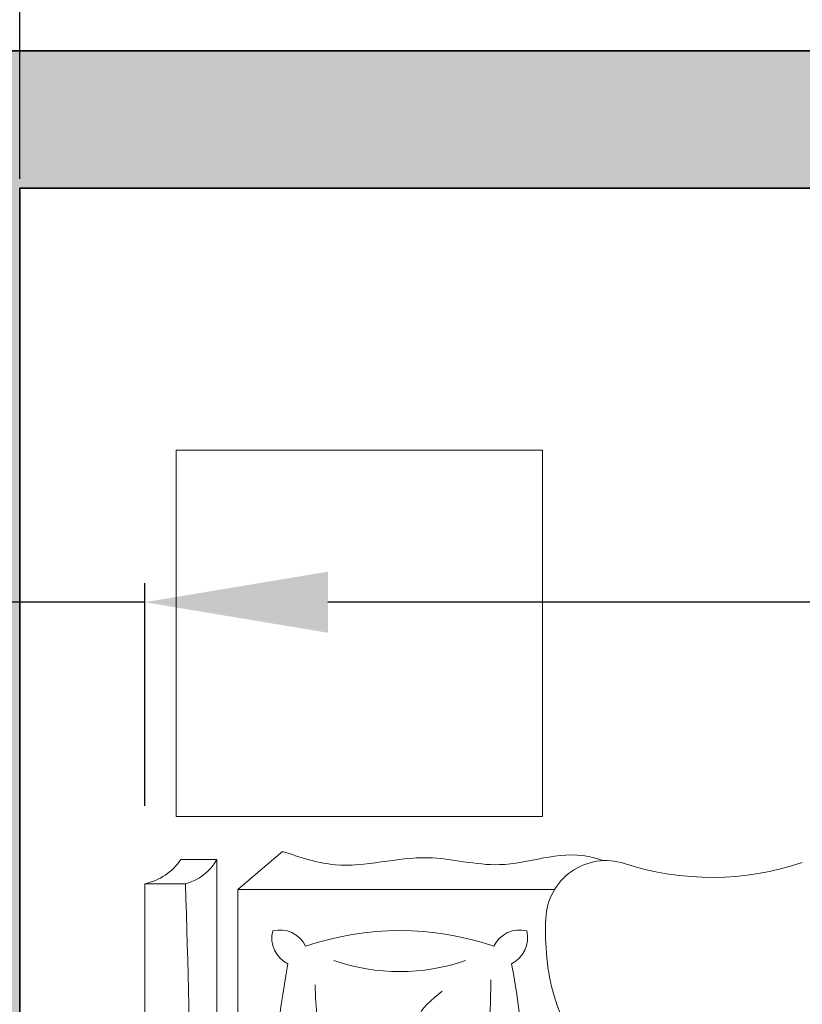
# Model space of a CAD drawing. Units: inches. Extents: x 2083 to 3317, y 1141 to 2115.
# Tile 98 of 256: x 2236 to 2287, y 1958 to 2023. Entities that reach past the tile are written whole.
import ezdxf

# ---------------------------------------------------------------- set-up
doc = ezdxf.new("R2010")
doc.units = ezdxf.units.IN
for name, color, linetype, lineweight in [('A-ANNO-DIMS', 2, 'Continuous', 18), ('A-FURN', 8, 'Continuous', 18), ('A-WALL', 7, 'Continuous', 35), ('www.cadblocksfree.com', 7, 'Continuous', 9)]:
    doc.layers.add(name, color=color, linetype=linetype, lineweight=lineweight)
doc.layers.add('A-WALL-PATT', color=251, linetype='Continuous', lineweight=13, true_color=0x636466)
doc.styles.get("Standard").update_dxf_attribs({"font": 'arial.ttf'})
doc.dimstyles.new('ISO-25', dxfattribs={"dimtxt": 12, "dimasz": 12, "dimexe": 1.25, "dimexo": 0.625, "dimtad": 1, "dimlunit": 3, "dimtxsty": 'Standard', "dimcen": 2.5, "dimadec": 0, "dimazin": 0, "dimtfac": 1, "dimtmove": 0, "dimatfit": 3, "dimfxl": 1, "dimarcsym": 0})

# ---------------------------------------------------------------- blocks, each defined once
blk = doc.blocks.new('bed')
at = {"layer": 'www.cadblocksfree.com', "ltscale": 0.2}
for p, q in [((3426.763, 1473.586), (3426.763, 1476.249)), ((3426.379, 1470.154), (3428.883, 1467.22))]:
    blk.add_line(p, q, dxfattribs=at)
for points in [[(3426.763, 1476.249), (3363.002, 1476.249)], [(3417.573, 1471.524), (3428.347, 1471.524), (3428.347, 1473.886)], [(3426.379, 1449.413), (3426.379, 1470.154), (3363.387, 1470.154), (3363.387, 1447.076)]]:
    blk.add_lwpolyline(points, dxfattribs=at)
for centre, radius, start, end in [((3430.432, 1476.997), 3.744, 191.5225, 236.17289), ((3394.883, 2431.358), 958.303, 268.093559, 271.906441), ((3429.921, 1474.373), 3.255, 194.0061, 241.08242), ((3410.752, 1409.187), 58.677, 79.42346, 100.57654), ((3423.206, 1466.054), 1.87, 75.51665, 154.20995), ((3421.863, 1467.396), 1.87, 295.79005, 14.48335), ((3404.477, 1459.547), 19.215, 341.28525, 18.71475), ((3434.35, 1459.547), 13.338, 161.15984, 198.84016), ((3421.863, 1451.698), 1.87, 345.51665, 64.20995), ((3410.752, 1509.907), 58.677, 259.42346, 280.57654), ((3423.206, 1453.041), 1.87, 205.79005, 284.48335), ((3424.339, 1446.045), 3.937, 342.05113, 87.98513), ((3445.776, 1439.101), 18.596, 162.05113, 198.56572)]:
    blk.add_arc(centre, radius, start, end, dxfattribs=at)
for points, knots in [([(3428.883, 1467.22), (3428.494, 1466.08), (3427.438, 1462.983), (3429.036, 1458.154), (3427.377, 1452.621), (3429.083, 1448.872), (3428.374, 1446.522), (3428.273, 1446.192)], [0, 0, 0, 0, 0.0901802, 0.2449351, 0.3646438, 0.5132331, 0.5378548, 0.5378548, 0.5378548, 0.5378548]), ([(3420.141, 1465.083), (3418.661, 1465.041), (3416.141, 1464.969), (3414.502, 1462.52), (3413.283, 1462.165), (3413.011, 1462.086)], [0, 0, 0, 0, 4.163459, 7.093919, 7.934624, 7.934624, 7.934624, 7.934624]), ([(3419.716, 1456.774), (3419.174, 1457.459), (3418.052, 1458.876), (3415.084, 1457.893), (3413.26, 1458.594), (3412.241, 1458.985)], [0, 0, 0, 0, 2.388143, 4.935423, 8.166198, 8.166198, 8.166198, 8.166198]), ([(3420.479, 1453.579), (3418.77, 1453.599), (3415.179, 1453.639), (3412.269, 1455.762), (3410.745, 1456.874)], [0, 0, 0, 0, 5.002087, 10.507046, 10.507046, 10.507046, 10.507046]), ([(3409.943, 1443.853), (3413.12, 1445.837), (3417.433, 1449.66), (3422.724, 1450.042), (3424.477, 1449.98)], [1.3582378, 1.3582378, 1.3582378, 1.3582378, 1.6381418, 1.7706953, 1.7706953, 1.7706953, 1.7706953])]:
    blk.add_open_spline(points, degree=3, knots=knots, dxfattribs=at)
blk = doc.blocks.new('*D20')
at = {"layer": 'A-ANNO-DIMS', "color": 0, "lineweight": -2, "transparency": 16777216}
for p, q in [((2244.15, 1971.316), (2244.15, 1985.902)), ((2337.22, 1971.316), (2337.22, 1985.902)), ((2244.15, 1984.652), (2119.159, 1984.652)), ((2325.22, 1984.652), (2256.15, 1984.652))]:
    blk.add_line(p, q, dxfattribs=at)
at = {"layer": 'A-ANNO-DIMS', "color": 0, "transparency": 16777216}
for points in [[(2256.15, 1986.652), (2256.15, 1982.652), (2244.15, 1984.652)], [(2325.22, 1986.652), (2325.22, 1982.652), (2337.22, 1984.652)]]:
    blk.add_solid(points, dxfattribs=at)
at = {"layer": 'Defpoints', "color": 0, "transparency": 16777216}
for p in [(2244.15, 1984.652), (2244.15, 1970.691), (2337.22, 1970.691)]:
    blk.add_point(p, dxfattribs=at)
at = {"layer": 'A-ANNO-DIMS', "color": 0, "transparency": 16777216, "insert": (2175.654, 1991.404), "char_height": 12, "attachment_point": 5}
blk.add_mtext('BED 7\'-9" TYP.', dxfattribs=at)
blk = doc.blocks.new('*D36')
at = {"layer": 'A-ANNO-DIMS', "color": 0, "lineweight": -2, "transparency": 16777216}
for p, q in [((2235.96, 2012.386), (2235.96, 2074.361)), ((2471.46, 2012.386), (2471.46, 2074.361)), ((2247.96, 2073.111), (2459.46, 2073.111))]:
    blk.add_line(p, q, dxfattribs=at)
at = {"layer": 'A-ANNO-DIMS', "color": 0, "transparency": 16777216}
for points in [[(2247.96, 2075.111), (2247.96, 2071.111), (2235.96, 2073.111)], [(2459.46, 2075.111), (2459.46, 2071.111), (2471.46, 2073.111)]]:
    blk.add_solid(points, dxfattribs=at)
at = {"layer": 'Defpoints', "color": 0, "transparency": 16777216}
for p in [(2471.46, 2073.111), (2235.96, 2011.761), (2471.46, 2011.761)]:
    blk.add_point(p, dxfattribs=at)
at = {"layer": 'A-ANNO-DIMS', "color": 0, "transparency": 16777216, "insert": (2353.71, 2079.941), "char_height": 12, "attachment_point": 5}
blk.add_mtext('19\'-7 1/2"', dxfattribs=at)

msp = doc.modelspace()

# ---------------------------------------------------------------- hatches: boundary and pattern name
at = {"layer": 'A-WALL-PATT'}
h = msp.add_hatch(color=256, dxfattribs=at)
h.dxf.hatch_style = 1
h.paths.add_polyline_path([(3126.96, 2020.761), (2748.96, 2020.761), (2604.96, 2020.761), (2226.96, 2020.761), (2226.96, 1702.761), (2466.96, 1702.761), (2466.96, 1582.761), (2418.96, 1582.761), (2418.96, 1477.761), (2226.96, 1477.761), (2226.96, 1263.261), (2544.96, 1263.261), (2544.96, 1411.761), (2604.96, 1411.761), (2685.96, 1411.761), (2685.96, 1420.761), (2604.96, 1420.761), (2604.96, 1573.761), (2604.96, 1702.761), (2604.96, 2011.761), (2748.96, 2011.761), (2748.96, 1702.761), (2862.96, 1702.761), (2862.96, 1621.761), (2871.96, 1621.761), (2871.96, 1702.761), (2883.96, 1702.761), (2883.96, 1706.939, -0.026459), (2883.96, 1711.761), (2757.96, 1711.761), (2757.96, 1807.761), (2787.96, 1807.761), (2787.96, 1812.261), (2757.96, 1812.261), (2757.96, 2011.761), (2877.96, 2011.761), (2877.96, 1812.261), (2847.96, 1812.261), (2847.96, 1807.761), (2889.836, 1807.761), (2889.836, 1812.261), (2882.46, 1812.261), (2882.46, 2011.761), (3117.96, 2011.761), (3117.96, 1812.261), (2937.836, 1812.261), (2937.836, 1807.761), (2995.71, 1807.761), (2995.71, 1796.118), (3000.21, 1796.118), (3000.21, 1807.761), (3117.96, 1807.761), (3117.96, 1711.761), (3000.21, 1711.761), (3000.21, 1760.118), (2998.573, 1760.118, -0.020711), (2995.71, 1760.118), (2995.71, 1711.761), (2931.96, 1711.761), (2931.96, 1702.761), (3126.96, 1702.761)])
h.paths.add_polyline_path([(2471.46, 2011.761), (2471.46, 1810.011), (2462.717, 1810.011), (2462.717, 1805.511), (2505.96, 1805.511), (2505.96, 1810.011), (2475.96, 1810.011), (2475.96, 2011.761), (2595.96, 2011.761), (2595.96, 1810.011), (2565.96, 1810.011), (2565.96, 1805.511), (2595.96, 1805.511), (2595.96, 1711.761), (2235.96, 1711.761), (2235.96, 1805.511), (2353.71, 1805.511), (2353.71, 1796.054), (2358.21, 1796.054), (2358.21, 1805.511), (2414.717, 1805.511), (2414.717, 1810.011), (2235.96, 1810.011), (2235.96, 2011.761)], flags=16)
h.paths.add_polyline_path([(2270.205, 1994.61), (2270.205, 1970.61), (2246.205, 1970.61), (2246.205, 1994.61)], flags=0)
edge = h.paths.add_edge_path(flags=0)
edge.add_ellipse((2332.027, 1899.798), major_axis=(-3.043, 3.043), ratio=0.168252, start_angle=-161.33217, end_angle=-156.30711, ccw=False)
edge.add_ellipse((2333.082, 1898.744), major_axis=(-1.055, 1.055), ratio=0.453532, start_angle=-123.37102, end_angle=-94.15911)
edge = h.paths.add_edge_path(flags=0)
edge.add_ellipse((2332.027, 1968.876), major_axis=(3.043, 3.043), ratio=0.168252, start_angle=18.66783, end_angle=23.69289)
edge.add_spline(control_points=[(2332.926, 1970.691), (2332.227, 1970.336), (2330.894, 1969.659), (2328.413, 1970.932), (2327.204, 1967.749), (2324.71, 1969.956), (2322.533, 1967.012), (2320.013, 1971.296), (2317.68, 1968.158), (2316.041, 1967.102), (2315.427, 1966.81)], knot_values=[0, 0, 0, 0, 2.267059, 4.324559, 6.685584, 8.878641, 11.121502, 14.300359, 17.755284, 19.732645, 19.732645, 19.732645, 19.732645], degree=3, periodic=0)
edge.add_ellipse((2332.027, 1968.876), major_axis=(3.043, 3.043), ratio=0.168252, start_angle=18.66783, end_angle=23.69289, ccw=False)
edge.add_ellipse((2333.082, 1969.931), major_axis=(1.055, 1.055), ratio=0.453532, start_angle=56.62898, end_angle=85.84089, ccw=False)
edge = h.paths.add_edge_path(flags=0)
edge.add_spline(control_points=[(2296.428, 1967.988), (2293.628, 1965.336), (2287.704, 1959.727), (2299.744, 1949.996), (2294.533, 1935.669), (2290.573, 1920.604), (2293.394, 1909.974), (2296.185, 1904.967)], knot_values=[0.099185, 0.099185, 0.099185, 0.099185, 0.345301, 0.619822, 0.982653, 1.386093, 1.810555, 1.810555, 1.810555, 1.810555], degree=3, periodic=0)
edge.add_spline(control_points=[(2296.185, 1904.967), (2297.384, 1902.619), (2298.001, 1901.949), (2298.553, 1901.468)], knot_values=[0.006246, 0.006246, 0.006246, 0.006246, 0.055476, 0.055476, 0.055476, 0.055476], degree=3, periodic=0)
edge.add_spline(control_points=[(2298.553, 1901.468), (2297.259, 1900.923), (2295.225, 1900.232), (2293.06, 1900.614), (2292.101, 1900.788), (2292.09, 1900.791)], knot_values=[0.312835, 0.312835, 0.312835, 0.312835, 0.40178, 0.474987, 0.475903, 0.475903, 0.475903, 0.475903], degree=3, periodic=0)
edge.add_arc((2292.794, 1904.664), 3.937, 215.4209, 259.69818, ccw=False)
edge.add_spline(control_points=[(2289.585, 1902.382), (2289.477, 1902.535), (2289.368, 1902.688), (2289.261, 1902.841)], knot_values=[0.102872, 0.102872, 0.102872, 0.102872, 0.116896, 0.116896, 0.116896, 0.116896], degree=3, periodic=0)
edge.add_spline(control_points=[(2289.261, 1902.841), (2288.687, 1902.55), (2287.64, 1902.02), (2285.881, 1901.874), (2283.853, 1901.504), (2281.72, 1899.711), (2278.467, 1899.493), (2276.157, 1901.883), (2272.259, 1899.804), (2267.778, 1901.843), (2262.244, 1900.184), (2257.415, 1901.782), (2254.318, 1900.726), (2253.178, 1900.337)], knot_values=[0, 0, 0, 0, 1.907977, 3.477176, 5.261074, 7.972851, 11.680248, 13.717921, 16.939592, 22.789562, 27.502503, 33.595215, 37.145618, 37.145618, 37.145618, 37.145618], degree=3, periodic=0)
edge.add_line((2253.178, 1900.337), (2250.244, 1902.841))
edge.add_line((2250.244, 1902.841), (2250.244, 1965.833))
edge.add_line((2250.244, 1965.833), (2253.178, 1968.337))
edge.add_spline(control_points=[(2253.178, 1968.337), (2254.318, 1967.948), (2257.415, 1966.892), (2262.244, 1968.49), (2267.778, 1966.831), (2271.527, 1968.537), (2273.876, 1967.828), (2274.207, 1967.728)], knot_values=[0, 0, 0, 0, 0.09018, 0.244935, 0.364644, 0.513233, 0.537855, 0.537855, 0.537855, 0.537855], degree=3, periodic=0)
edge.add_arc((2274.353, 1963.793), 3.937, 72.05113, 92.12795, ccw=False)
edge.add_arc((2281.297, 1985.23), 18.596, 252.05113, 288.56572)
edge.add_arc((2292.317, 1956.029), 12.646, 71.02679, 113.77822, ccw=False)
edge = h.paths.add_edge_path(flags=0)
edge.add_spline(control_points=[(2274.899, 1951.856), (2275.066, 1951.617), (2275.233, 1951.377), (2275.398, 1951.136)], knot_values=[1.409916, 1.409916, 1.409916, 1.409916, 1.43159, 1.43159, 1.43159, 1.43159], degree=3, periodic=0)
edge.add_spline(control_points=[(2275.398, 1951.136), (2275.792, 1950.562), (2276.179, 1949.984), (2276.546, 1949.397)], knot_values=[1.358238, 1.358238, 1.358238, 1.358238, 1.409916, 1.409916, 1.409916, 1.409916], degree=3, periodic=0)
edge.add_line((2276.546, 1949.397), (2277.437, 1947.862))
edge.add_spline(control_points=[(2277.437, 1947.862), (2276.304, 1945.673), (2274.64, 1942.427), (2274.632, 1938.094), (2272.799, 1930.852), (2274.356, 1943.897), (2275.948, 1947.923), (2276.546, 1949.397)], knot_values=[0.005632, 0.005632, 0.005632, 0.005632, 0.186014, 0.266002, 0.357087, 0.59639, 0.739732, 0.739732, 0.739732, 0.739732], degree=3, periodic=0)
edge.add_spline(control_points=[(2276.546, 1949.397), (2276.179, 1949.984), (2275.792, 1950.562), (2275.398, 1951.136)], knot_values=[1.358238, 1.358238, 1.358238, 1.358238, 1.409916, 1.409916, 1.409916, 1.409916], degree=3, periodic=0)
edge.add_spline(control_points=[(2275.398, 1951.136), (2274.943, 1950.08), (2274.208, 1948.025), (2273.935, 1944.851), (2272.469, 1937.627), (2273.466, 1945.696), (2274.701, 1951.059), (2274.899, 1951.856)], knot_values=[0.104364, 0.104364, 0.104364, 0.104364, 0.189636, 0.269624, 0.36071, 0.600013, 0.644622, 0.644622, 0.644622, 0.644622], degree=3, periodic=0)
h.paths.add_polyline_path([(2269.168, 1963.128, -0.357527), (2268.171, 1960.976, -0.092561), (2268.171, 1939.436, -0.357527), (2269.168, 1937.285, -0.357527), (2267.016, 1938.282, -0.164785), (2254.686, 1938.282, -0.357527), (2252.534, 1937.285, -0.357527), (2253.531, 1939.436, -0.092561), (2253.531, 1960.976, -0.357527), (2252.534, 1963.128, -0.357527), (2254.686, 1962.131, -0.164785), (2267.016, 1962.131, -0.357527)], flags=0)
h.paths.add_polyline_path([(2248.874, 1967.802), (2248.874, 1957.028), (2249.458, 1957.028), (2249.458, 1911.647), (2248.874, 1911.647), (2248.874, 1900.873), (2246.512, 1900.873, 0.197327), (2244.15, 1902.457), (2244.15, 1966.218, 0.197327), (2246.512, 1967.802)], flags=0)
h.paths.add_polyline_path([(2269.168, 1931.389, -0.357527), (2268.171, 1929.238, -0.092561), (2268.171, 1907.698, -0.357527), (2269.168, 1905.547, -0.357527), (2267.016, 1906.544, -0.164785), (2254.686, 1906.544, -0.357527), (2252.534, 1905.547, -0.357527), (2253.531, 1907.698, -0.092561), (2253.531, 1929.238, -0.357527), (2252.534, 1931.389, -0.357527), (2254.686, 1930.392, -0.164785), (2267.016, 1930.392, -0.357527)], flags=0)
edge = h.paths.add_edge_path(flags=0)
edge.add_spline(control_points=[(2276.197, 1906.724), (2276.168, 1909.029), (2276.114, 1913.372), (2270.598, 1924.925), (2273.905, 1919.013), (2275.922, 1916.262), (2275.475, 1912.402), (2277.258, 1910.381), (2276.696, 1908.225), (2276.646, 1906.813), (2276.618, 1906.008)], knot_values=[0, 0, 0, 0, 8.61026, 16.221274, 18.843057, 23.804898, 27.440828, 29.356102, 31.203478, 33.650687, 33.650687, 33.650687, 33.650687], degree=3, periodic=0)
edge.add_spline(control_points=[(2276.618, 1906.008), (2276.623, 1905.624), (2276.498, 1904.629), (2275.442, 1903.855), (2274.937, 1903.08), (2274.859, 1902.841)], knot_values=[0.156488, 0.156488, 0.156488, 0.156488, 0.184398, 0.231376, 0.250598, 0.250598, 0.250598, 0.250598], degree=3, periodic=0)
edge.add_line((2274.859, 1902.841), (2276.506, 1902.841))
edge.add_spline(control_points=[(2276.506, 1902.841), (2276.788, 1903.085), (2277.665, 1904.125), (2278.25, 1904.341), (2277.654, 1908.527), (2278.156, 1906.228), (2278.1, 1905.286), (2278.847, 1904.069), (2277.857, 1903.415), (2277.874, 1902.991), (2277.904, 1902.841)], knot_values=[0.059574, 0.059574, 0.059574, 0.059574, 0.080753, 0.103741, 0.16972, 0.176036, 0.207137, 0.240474, 0.262341, 0.27366, 0.27366, 0.27366, 0.27366], degree=3, periodic=0)
edge.add_line((2277.904, 1902.841), (2280.03, 1902.841))
edge.add_spline(control_points=[(2280.03, 1902.841), (2279.888, 1903.088), (2279.499, 1903.982), (2280.152, 1905.939), (2278.104, 1909.658), (2279.762, 1907.185), (2280.328, 1904.875), (2280.485, 1903.49), (2281.463, 1903.249), (2281.758, 1902.936), (2281.834, 1902.841)], knot_values=[0.013856, 0.013856, 0.013856, 0.013856, 0.034874, 0.088867, 0.107879, 0.126738, 0.158714, 0.193757, 0.217487, 0.226722, 0.226722, 0.226722, 0.226722], degree=3, periodic=0)
edge.add_spline(control_points=[(2281.834, 1902.841), (2281.788, 1902.827), (2281.647, 1902.783), (2281.396, 1902.859), (2281.088, 1902.985), (2280.721, 1903.061), (2280.333, 1903.026), (2280.125, 1902.899), (2280.03, 1902.841)], knot_values=[0, 0, 0, 0, 0.14413, 0.435517, 0.749276, 1.153046, 1.548371, 1.878348, 1.878348, 1.878348, 1.878348], degree=3, periodic=0)
edge.add_line((2280.03, 1902.841), (2277.904, 1902.841))
edge.add_spline(control_points=[(2277.904, 1902.841), (2277.893, 1902.796), (2277.865, 1902.68), (2277.607, 1902.687), (2277.274, 1902.801), (2276.838, 1902.62), (2276.584, 1902.789), (2276.506, 1902.841)], knot_values=[0, 0, 0, 0, 0.127189, 0.326199, 0.628009, 1.24357, 1.515331, 1.515331, 1.515331, 1.515331], degree=3, periodic=0)
edge.add_line((2276.506, 1902.841), (2274.859, 1902.841))
edge.add_spline(control_points=[(2274.859, 1902.841), (2274.814, 1902.899), (2274.725, 1903.013), (2274.493, 1903.119), (2274.244, 1902.961), (2273.937, 1903.185), (2273.614, 1902.983), (2273.408, 1902.883), (2273.322, 1902.841)], knot_values=[0, 0, 0, 0, 0.21843, 0.436957, 0.687977, 0.990379, 1.398396, 1.69185, 1.69185, 1.69185, 1.69185], degree=3, periodic=0)
edge.add_spline(control_points=[(2273.322, 1902.841), (2273.617, 1903.446), (2274.274, 1904.538), (2276.027, 1904.574), (2276.207, 1906.584), (2276.197, 1906.724)], knot_values=[0.012227, 0.012227, 0.012227, 0.012227, 0.059472, 0.106218, 0.134458, 0.134458, 0.134458, 0.134458], degree=3, periodic=0)
h.paths.add_polyline_path([(2270.776, 1897.79), (2270.776, 1873.79), (2246.776, 1873.79), (2246.776, 1897.79)], flags=0)
h.paths.add_polyline_path([(2353.71, 1760.005), (2353.71, 1760.054), (2358.21, 1760.054, -0.033729)], flags=0)
h.paths.add_polyline_path([(2321.819, 1737.529), (2341.995, 1737.529, -0.414214), (2343.203, 1736.321), (2343.203, 1721.021, -0.414214), (2341.995, 1719.813), (2321.819, 1719.813, -0.414214), (2320.611, 1721.021), (2320.611, 1736.321, -0.414214)], flags=0)
h.paths.add_polyline_path([(2324.235, 1736.321), (2339.579, 1736.321, -0.414214), (2341.995, 1733.905), (2341.995, 1725.45, -0.414214), (2339.579, 1723.034), (2333.681, 1723.034), (2333.845, 1722.045, -0.870646), (2335.425, 1721.826, -0.767327), (2333.923, 1721.423), (2331.291, 1721.423, -0.767327), (2329.788, 1721.826, -0.870646), (2331.368, 1722.045), (2331.533, 1723.034), (2324.235, 1723.034, -0.414214), (2321.819, 1725.45), (2321.819, 1733.905, -0.414214)], flags=0)
h.paths.add_polyline_path([(2570.484, 1928.615), (2589.684, 1928.615), (2590.169, 1928.615), (2590.169, 1904.993), (2570.484, 1904.993)], flags=0)
h.paths.add_polyline_path([(2574.447, 1927.264, -1), (2572.829, 1927.264, -1)], flags=0)
h.paths.add_polyline_path([(2573.09, 1926.941), (2573.925, 1927.776), (2574.148, 1927.553), (2573.313, 1926.718)], flags=0)
h.paths.add_polyline_path([(2578.779, 1919.73, -1), (2571.592, 1919.73, -1)], flags=0)
h.paths.add_polyline_path([(2578.385, 1919.73, -1), (2571.985, 1919.73, -1)], flags=0)
h.paths.add_polyline_path([(2331.596, 1729.476, -1), (2333.618, 1729.476, -1)], flags=0)
h.paths.add_polyline_path([(2578.034, 1927.264, -1), (2576.416, 1927.264, -1)], flags=0)
h.paths.add_polyline_path([(2576.689, 1927.531), (2576.912, 1927.754), (2577.747, 1926.919), (2577.524, 1926.696)], flags=0)
h.paths.add_polyline_path([(2578.139, 1909.86, -1), (2572.232, 1909.86, -1)], flags=0)
h.paths.add_polyline_path([(2577.745, 1909.86, -1), (2572.625, 1909.86, -1)], flags=0)
h.paths.add_polyline_path([(2583.798, 1927.264, -1), (2582.179, 1927.264, -1)], flags=0)
h.paths.add_polyline_path([(2582.719, 1927.754), (2583.554, 1926.919), (2583.331, 1926.696), (2582.496, 1927.531)], flags=0)
h.paths.add_polyline_path([(2582.496, 1927.531), (2582.719, 1927.754), (2583.554, 1926.919), (2583.331, 1926.696)], flags=0)
h.paths.add_polyline_path([(2587.739, 1920.53, -1), (2581.832, 1920.53, -1)], flags=0)
h.paths.add_polyline_path([(2587.345, 1920.53, -1), (2582.225, 1920.53, -1)], flags=0)
h.paths.add_polyline_path([(2587.385, 1927.264, -1), (2585.766, 1927.264, -1)], flags=0)
h.paths.add_polyline_path([(2586.082, 1926.98), (2586.917, 1927.815), (2587.14, 1927.593), (2586.305, 1926.758)], flags=0)
h.paths.add_polyline_path([(2588.379, 1910.66, -1), (2581.192, 1910.66, -1)], flags=0)
h.paths.add_polyline_path([(2587.985, 1910.66, -1), (2581.585, 1910.66, -1)], flags=0)
h.paths.add_polyline_path([(2417.168, 1729.478), (2437.344, 1729.478, -0.414214), (2438.552, 1728.27), (2438.552, 1712.969, -0.414214), (2437.344, 1711.761), (2417.168, 1711.761, -0.414214), (2415.96, 1712.969), (2415.96, 1728.27, -0.414214)], flags=0)
h.paths.add_polyline_path([(2419.584, 1728.27), (2434.928, 1728.27, -0.414214), (2437.344, 1725.854), (2437.344, 1717.398, -0.414214), (2434.928, 1714.983), (2429.029, 1714.983), (2429.194, 1713.994, -0.870646), (2430.774, 1713.775, -0.767327), (2429.271, 1713.372), (2426.64, 1713.372, -0.767327), (2425.137, 1713.775, -0.870646), (2426.717, 1713.994), (2426.882, 1714.983), (2419.584, 1714.983, -0.414214), (2417.168, 1717.398), (2417.168, 1725.854, -0.414214)], flags=0)
h.paths.add_polyline_path([(2419.584, 1728.27), (2434.928, 1728.27, -0.414214), (2437.344, 1725.854), (2437.344, 1717.398, -0.414214), (2434.928, 1714.983), (2429.029, 1714.983), (2428.358, 1719.009), (2427.553, 1719.009), (2426.882, 1714.983), (2419.584, 1714.983, -0.414214), (2417.168, 1717.398), (2417.168, 1725.854, -0.414214)], flags=0)
h.paths.add_polyline_path([(2426.944, 1721.425, -1), (2428.967, 1721.425, -1)], flags=0)
h.paths.add_polyline_path([(2475.96, 1702.761), (2595.96, 1702.761), (2595.96, 1582.761), (2475.96, 1582.761)], flags=16)
h.paths.add_polyline_path([(2427.96, 1573.761), (2595.96, 1573.761), (2595.96, 1468.761), (2595.96, 1420.761), (2384.46, 1420.761), (2384.46, 1468.761), (2427.96, 1468.761)], flags=16)
h.paths.add_polyline_path([(2379.96, 1468.761), (2379.96, 1420.761), (2235.96, 1420.761), (2235.96, 1468.761)], flags=16)
h.paths.add_polyline_path([(2317.816, 1466.696), (2337.992, 1466.696, -0.414214), (2339.2, 1465.488), (2339.2, 1450.187, -0.414214), (2337.992, 1448.979), (2317.816, 1448.979, -0.414214), (2316.608, 1450.187), (2316.608, 1465.488, -0.414214)], flags=0)
h.paths.add_polyline_path([(2320.232, 1465.488), (2335.576, 1465.488, -0.414214), (2337.992, 1463.072), (2337.992, 1454.616, -0.414214), (2335.576, 1452.2), (2329.677, 1452.2), (2329.842, 1451.212, -0.870646), (2331.422, 1450.992, -0.767327), (2329.92, 1450.59), (2327.288, 1450.59, -0.767327), (2325.785, 1450.992, -0.870646), (2327.365, 1451.212), (2327.53, 1452.2), (2320.232, 1452.2, -0.414214), (2317.816, 1454.616), (2317.816, 1463.072, -0.414214)], flags=0)
h.paths.add_polyline_path([(2320.232, 1465.488), (2335.576, 1465.488, -0.414214), (2337.992, 1463.072), (2337.992, 1454.616, -0.414214), (2335.576, 1452.2), (2329.677, 1452.2), (2329.006, 1456.227), (2328.201, 1456.227), (2327.53, 1452.2), (2320.232, 1452.2, -0.414214), (2317.816, 1454.616), (2317.816, 1463.072, -0.414214)], flags=0)
h.paths.add_polyline_path([(2327.593, 1458.643, -1), (2329.615, 1458.643, -1)], flags=0)
h.paths.add_polyline_path([(2244.412, 1433.34), (2241.921, 1433.34, -0.414214), (2240.018, 1435.244), (2240.018, 1440.953, -0.414211), (2241.921, 1442.856), (2244.412, 1442.856, -1.976472)], flags=0)
h.paths.add_polyline_path([(2245.357, 1434.398, -0.414214), (2245.357, 1441.799, -2.144098)], flags=0)
h.paths.add_polyline_path([(2535.96, 1416.261), (2535.96, 1272.261), (2235.96, 1272.261), (2235.96, 1416.261)], flags=16)
h.paths.add_polyline_path([(2260.12, 1384.293), (2260.12, 1362.039), (2237.865, 1362.039), (2237.865, 1384.293)], flags=0)
edge = h.paths.add_edge_path(flags=0)
edge.add_line((2318.252, 1362.093), (2318.146, 1362.001))
edge.add_ellipse((2317.445, 1360.431), major_axis=(2.822, 2.822), ratio=0.168252, start_angle=18.66783, end_angle=20.94813, ccw=False)
edge.add_ellipse((2318.423, 1361.409), major_axis=(0.978, 0.978), ratio=0.453532, start_angle=56.62898, end_angle=70.2262, ccw=False)
edge = h.paths.add_edge_path(flags=0)
edge.add_line((2319.107, 1295.571), (2319.015, 1295.677))
edge.add_ellipse((2317.445, 1296.378), major_axis=(-2.822, 2.822), ratio=0.168252, start_angle=-161.33217, end_angle=-159.05187, ccw=False)
edge.add_ellipse((2318.423, 1295.4), major_axis=(-0.978, 0.978), ratio=0.453532, start_angle=-123.37102, end_angle=-109.7738)
edge = h.paths.add_edge_path(flags=0)
edge.add_spline(control_points=[(2284.21, 1301.17), (2284.581, 1300.445), (2284.891, 1299.892), (2285.16, 1299.461)], knot_values=[0.039066, 0.039066, 0.039066, 0.039066, 0.055476, 0.055476, 0.055476, 0.055476], degree=3, periodic=0)
edge.add_line((2285.16, 1299.461), (2284.21, 1301.17))
edge = h.paths.add_edge_path(flags=0)
edge.add_line((2280.412, 1297.298), (2283.37, 1297.036))
edge.add_line((2283.37, 1297.036), (2286.406, 1297.926))
edge.add_spline(control_points=[(2286.406, 1297.926), (2285.305, 1297.463), (2284.345, 1297.129), (2283.37, 1297.036)], knot_values=[0.394369, 0.394369, 0.394369, 0.394369, 0.475903, 0.475903, 0.475903, 0.475903], degree=3, periodic=0)
edge.add_spline(control_points=[(2283.37, 1297.036), (2283.281, 1297.028), (2282.316, 1296.957), (2281.313, 1297.134), (2280.423, 1297.296), (2280.412, 1297.298)], knot_values=[0.312835, 0.312835, 0.312835, 0.312835, 0.320246, 0.393453, 0.394369, 0.394369, 0.394369, 0.394369], degree=3, periodic=0)
edge = h.paths.add_edge_path(flags=0)
edge.add_line((2284.436, 1359.607), (2280.446, 1355.328))
edge.add_line((2280.446, 1355.328), (2279.58, 1351.018))
edge.add_line((2279.58, 1351.018), (2282.413, 1346.58))
edge.add_spline(control_points=[(2282.413, 1346.58), (2283.153, 1345.589), (2284.253, 1344.029), (2284.801, 1342.387), (2284.935, 1341.806)], knot_values=[1.240098, 1.240098, 1.240098, 1.240098, 1.332892, 1.382712, 1.382712, 1.382712, 1.382712], degree=3, periodic=0)
edge.add_spline(control_points=[(2284.935, 1341.806), (2285.319, 1340.141), (2285.233, 1338.409), (2284.91, 1336.654)], knot_values=[1.097484, 1.097484, 1.097484, 1.097484, 1.240098, 1.240098, 1.240098, 1.240098], degree=3, periodic=0)
edge.add_spline(control_points=[(2284.91, 1336.654), (2284.587, 1334.899), (2284.027, 1333.12), (2283.463, 1331.361)], knot_values=[0.95487, 0.95487, 0.95487, 0.95487, 1.097484, 1.097484, 1.097484, 1.097484], degree=3, periodic=0)
edge.add_line((2283.463, 1331.361), (2281.89, 1326.153))
edge.add_line((2281.89, 1326.153), (2280.756, 1321.056))
edge.add_line((2280.756, 1321.056), (2280.299, 1316.002))
edge.add_line((2280.299, 1316.002), (2280.716, 1310.95))
edge.add_line((2280.716, 1310.95), (2282.028, 1305.972))
edge.add_line((2282.028, 1305.972), (2284.21, 1301.17))
edge.add_spline(control_points=[(2284.21, 1301.17), (2283.341, 1302.73), (2282.612, 1304.336), (2282.028, 1305.972)], knot_values=[0.099185, 0.099185, 0.099185, 0.099185, 0.241799, 0.241799, 0.241799, 0.241799], degree=3, periodic=0)
edge.add_spline(control_points=[(2282.028, 1305.972), (2281.444, 1307.608), (2281.005, 1309.273), (2280.716, 1310.95)], knot_values=[0.241799, 0.241799, 0.241799, 0.241799, 0.384413, 0.384413, 0.384413, 0.384413], degree=3, periodic=0)
edge.add_spline(control_points=[(2280.716, 1310.95), (2280.433, 1312.588), (2280.289, 1314.277), (2280.299, 1315.962), (2280.299, 1316.002)], knot_values=[0.384413, 0.384413, 0.384413, 0.384413, 0.523647, 0.527028, 0.527028, 0.527028, 0.527028], degree=3, periodic=0)
edge.add_spline(control_points=[(2280.299, 1316.002), (2280.312, 1317.687), (2280.478, 1319.368), (2280.756, 1321.056)], knot_values=[0.527028, 0.527028, 0.527028, 0.527028, 0.669642, 0.669642, 0.669642, 0.669642], degree=3, periodic=0)
edge.add_spline(control_points=[(2280.756, 1321.056), (2281.035, 1322.744), (2281.426, 1324.44), (2281.89, 1326.153)], knot_values=[0.669642, 0.669642, 0.669642, 0.669642, 0.812256, 0.812256, 0.812256, 0.812256], degree=3, periodic=0)
edge.add_spline(control_points=[(2281.89, 1326.153), (2282.264, 1327.533), (2282.788, 1329.262), (2283.353, 1331.018), (2283.463, 1331.361)], knot_values=[0.812256, 0.812256, 0.812256, 0.812256, 0.927087, 0.95487, 0.95487, 0.95487, 0.95487], degree=3, periodic=0)
edge.add_line((2283.463, 1331.361), (2284.91, 1336.654))
edge.add_line((2284.91, 1336.654), (2284.935, 1341.806))
edge.add_line((2284.935, 1341.806), (2282.413, 1346.58))
edge.add_spline(control_points=[(2282.413, 1346.58), (2281.275, 1348.104), (2280.078, 1349.57), (2279.58, 1351.018)], knot_values=[1.382712, 1.382712, 1.382712, 1.382712, 1.525326, 1.525326, 1.525326, 1.525326], degree=3, periodic=0)
edge.add_spline(control_points=[(2279.58, 1351.018), (2279.443, 1351.415), (2279.136, 1352.857), (2279.735, 1354.29), (2280.446, 1355.328)], knot_values=[1.525326, 1.525326, 1.525326, 1.525326, 1.564439, 1.667941, 1.667941, 1.667941, 1.667941], degree=3, periodic=0)
edge.add_spline(control_points=[(2280.446, 1355.328), (2281.426, 1356.758), (2282.931, 1358.183), (2284.436, 1359.607)], knot_values=[1.667941, 1.667941, 1.667941, 1.667941, 1.810555, 1.810555, 1.810555, 1.810555], degree=3, periodic=0)
edge.add_arc((2280.623, 1348.518), 11.726, 71.02679, 113.77822)
edge.add_arc((2270.405, 1375.595), 17.244, 252.05113, 288.56572, ccw=False)
edge.add_arc((2263.966, 1355.718), 3.651, 72.05113, 92.12795)
edge.add_arc((2263.966, 1355.718), 3.651, 92.12795, 177.98513)
edge.add_spline(control_points=[(2260.318, 1355.846), (2260.26, 1354.221), (2260.551, 1350.187), (2262.999, 1346.766), (2264.473, 1344.649)], knot_values=[1.43159, 1.43159, 1.43159, 1.43159, 1.564144, 1.770695, 1.770695, 1.770695, 1.770695], degree=3, periodic=0)
edge.add_line((2264.473, 1344.649), (2264.936, 1343.983))
edge.add_spline(control_points=[(2263.801, 1340.248), (2263.843, 1340.514), (2264.067, 1341.756), (2264.513, 1343.002), (2264.935, 1343.981)], knot_values=[0.53657, 0.53657, 0.53657, 0.53657, 0.559349, 0.644622, 0.644622, 0.644622, 0.644622], degree=3, periodic=0)
edge.add_spline(control_points=[(2264.935, 1343.981), (2265.118, 1343.715), (2265.299, 1343.448), (2265.477, 1343.179)], knot_values=[1.384077, 1.384077, 1.384077, 1.384077, 1.409916, 1.409916, 1.409916, 1.409916], degree=3, periodic=0)
edge.add_spline(control_points=[(2265.477, 1343.179), (2265.655, 1342.911), (2265.829, 1342.641), (2265.999, 1342.369)], knot_values=[1.358238, 1.358238, 1.358238, 1.358238, 1.384077, 1.384077, 1.384077, 1.384077], degree=3, periodic=0)
edge.add_line((2265.999, 1342.369), (2266.826, 1340.946))
edge.add_spline(control_points=[(2266.826, 1340.946), (2268.894, 1337.09), (2271.398, 1325.843), (2270.516, 1310.569), (2275.919, 1301.861), (2277.79, 1299.199)], knot_values=[0.116896, 0.116896, 0.116896, 0.116896, 0.472987, 1.050969, 1.313793, 1.313793, 1.313793, 1.313793], degree=3, periodic=0)
edge.add_spline(control_points=[(2277.79, 1299.199), (2277.839, 1299.128), (2277.889, 1299.057), (2277.94, 1298.987)], knot_values=[0.109884, 0.109884, 0.109884, 0.109884, 0.116896, 0.116896, 0.116896, 0.116896], degree=3, periodic=0)
edge.add_line((2277.94, 1298.987), (2277.789, 1299.199))
edge.add_spline(control_points=[(2277.789, 1299.199), (2277.257, 1298.929), (2276.286, 1298.438), (2275.039, 1298.334), (2274.383, 1298.239), (2274.215, 1298.209)], knot_values=[33.12187, 33.12187, 33.12187, 33.12187, 35.029056, 36.598255, 37.144827, 37.144827, 37.144827, 37.144827], degree=3, periodic=0)
edge.add_line((2274.215, 1298.209), (2273.073, 1297.893))
edge.add_spline(control_points=[(2273.073, 1297.893), (2272.323, 1297.58), (2271.039, 1296.511), (2269.248, 1296.226), (2268.423, 1296.375)], knot_values=[26.532584, 26.532584, 26.532584, 26.532584, 29.198919, 31.839101, 31.839101, 31.839101, 31.839101], degree=3, periodic=0)
edge.add_line((2268.423, 1296.375), (2263.879, 1297.458))
edge.add_spline(control_points=[(2263.879, 1297.458), (2263.556, 1297.359), (2261.86, 1296.839), (2260.239, 1297.282), (2258.933, 1297.516)], knot_values=[15.919551, 15.919551, 15.919551, 15.919551, 16.939592, 21.226067, 21.226067, 21.226067, 21.226067], degree=3, periodic=0)
edge.add_line((2258.933, 1297.516), (2254.055, 1297.329))
edge.add_spline(control_points=[(2254.055, 1297.329), (2253.756, 1297.296), (2252.114, 1297.165), (2250.462, 1297.544), (2249.13, 1297.668)], knot_values=[5.306517, 5.306517, 5.306517, 5.306517, 6.276435, 10.613034, 10.613034, 10.613034, 10.613034], degree=3, periodic=0)
edge.add_line((2249.13, 1297.668), (2244.332, 1296.878))
edge.add_line((2244.332, 1296.878), (2241.611, 1299.199))
edge.add_line((2241.611, 1299.199), (2241.611, 1357.609))
edge.add_line((2241.611, 1357.609), (2244.332, 1359.931))
edge.add_line((2244.332, 1359.931), (2252.729, 1359.543))
edge.add_spline(control_points=[(2252.729, 1359.543), (2252.871, 1359.546), (2253.306, 1359.548), (2253.74, 1359.514), (2254.032, 1359.482)], knot_values=[0.233291, 0.233291, 0.233291, 0.233291, 0.244935, 0.268927, 0.268927, 0.268927, 0.268927], degree=3, periodic=0)
edge.add_line((2254.032, 1359.482), (2259.587, 1359.416))
edge.add_spline(control_points=[(2259.587, 1359.416), (2260.677, 1359.629), (2262.073, 1359.897), (2263.524, 1359.459), (2263.83, 1359.366)], knot_values=[0.422516, 0.422516, 0.422516, 0.422516, 0.513233, 0.537855, 0.537855, 0.537855, 0.537855], degree=3, periodic=0)
edge.add_arc((2263.966, 1355.718), 3.651, 72.05113, 92.12795, ccw=False)
edge.add_arc((2270.405, 1375.595), 17.244, 252.05113, 288.56572)
edge.add_arc((2280.623, 1348.518), 11.726, 71.02679, 113.77822, ccw=False)
h.paths.add_polyline_path([(2240.341, 1359.435), (2240.341, 1349.444), (2240.882, 1349.444), (2240.882, 1307.365), (2240.341, 1307.365), (2240.341, 1297.374), (2238.15, 1297.374, 0.197327), (2235.96, 1298.843), (2235.96, 1357.966, 0.197327), (2238.15, 1359.435)], flags=0)
h.paths.add_polyline_path([(2259.158, 1355.101, -0.357527), (2258.233, 1353.106, -0.092561), (2258.233, 1333.133, -0.357527), (2259.158, 1331.138, -0.357527), (2257.163, 1332.062, -0.164785), (2245.729, 1332.062, -0.357527), (2243.735, 1331.138, -0.357527), (2244.659, 1333.133, -0.092561), (2244.659, 1353.106, -0.357527), (2243.735, 1355.101, -0.357527), (2245.729, 1354.176, -0.164785), (2257.163, 1354.176, -0.357527)], flags=0)
edge = h.paths.add_edge_path(flags=0)
edge.add_line((2265.999, 1342.369), (2266.826, 1340.946))
edge.add_line((2266.826, 1340.946), (2265.308, 1337.814))
edge.add_line((2265.308, 1337.814), (2264.358, 1334.653))
edge.add_line((2264.358, 1334.653), (2264.262, 1333.8))
edge.add_spline(control_points=[(2264.262, 1333.8), (2264.208, 1333.187), (2264.162, 1332.366), (2264.007, 1331.414), (2263.969, 1331.202)], knot_values=[0.464444, 0.464444, 0.464444, 0.464444, 0.516691, 0.531608, 0.531608, 0.531608, 0.531608], degree=3, periodic=0)
edge.add_spline(control_points=[(2263.969, 1331.202), (2263.775, 1330.119), (2263.424, 1328.791), (2263.257, 1328.531), (2263.234, 1328.515)], knot_values=[0.372682, 0.372682, 0.372682, 0.372682, 0.44885, 0.464444, 0.464444, 0.464444, 0.464444], degree=3, periodic=0)
edge.add_spline(control_points=[(2263.234, 1328.515), (2263.096, 1328.42), (2263.131, 1329.301), (2263.275, 1330.616)], knot_values=[0.280919, 0.280919, 0.280919, 0.280919, 0.372682, 0.372682, 0.372682, 0.372682], degree=3, periodic=0)
edge.add_spline(control_points=[(2263.275, 1330.616), (2263.419, 1331.93), (2263.672, 1333.677), (2263.97, 1335.315)], knot_values=[0.189157, 0.189157, 0.189157, 0.189157, 0.280919, 0.280919, 0.280919, 0.280919], degree=3, periodic=0)
edge.add_spline(control_points=[(2263.97, 1335.315), (2264.1, 1336.032), (2264.419, 1337.622), (2264.755, 1338.864), (2264.947, 1339.491)], knot_values=[0.097394, 0.097394, 0.097394, 0.097394, 0.137578, 0.189157, 0.189157, 0.189157, 0.189157], degree=3, periodic=0)
edge.add_spline(control_points=[(2264.947, 1339.491), (2265.29, 1340.606), (2265.644, 1341.494), (2265.999, 1342.369)], knot_values=[0.005632, 0.005632, 0.005632, 0.005632, 0.097394, 0.097394, 0.097394, 0.097394], degree=3, periodic=0)
h.paths.add_polyline_path([(2259.158, 1325.671, -0.357527), (2258.233, 1323.676, -0.092561), (2258.233, 1303.703, -0.357527), (2259.158, 1301.708, -0.357527), (2257.163, 1302.633, -0.164785), (2245.729, 1302.633, -0.357527), (2243.735, 1301.708, -0.357527), (2244.659, 1303.703, -0.092561), (2244.659, 1323.676, -0.357527), (2243.735, 1325.671, -0.357527), (2245.729, 1324.747, -0.164785), (2257.163, 1324.747, -0.357527)], flags=0)
edge = h.paths.add_edge_path(flags=0)
edge.add_spline(control_points=[(2261.709, 1317.311), (2261.679, 1317.418), (2261.762, 1317.389), (2262.491, 1316.09), (2262.962, 1315.301)], knot_values=[14.955861, 14.955861, 14.955861, 14.955861, 16.221274, 18.694826, 18.694826, 18.694826, 18.694826], degree=3, periodic=0)
edge.add_spline(control_points=[(2262.962, 1315.301), (2262.99, 1315.254), (2263.702, 1314.067), (2264.349, 1313.127), (2264.73, 1312.164)], knot_values=[18.694826, 18.694826, 18.694826, 18.694826, 18.843057, 22.433791, 22.433791, 22.433791, 22.433791], degree=3, periodic=0)
edge.add_spline(control_points=[(2264.73, 1312.164), (2264.876, 1311.796), (2265.177, 1310.77), (2265.143, 1309.559), (2265.248, 1308.824)], knot_values=[22.433791, 22.433791, 22.433791, 22.433791, 23.804898, 26.172756, 26.172756, 26.172756, 26.172756], degree=3, periodic=0)
edge.add_line((2265.248, 1308.824), (2265.851, 1307.172))
edge.add_spline(control_points=[(2265.851, 1307.172), (2266.065, 1306.822), (2266.384, 1306.332), (2266.424, 1305.781), (2266.42, 1305.611)], knot_values=[28.062562, 28.062562, 28.062562, 28.062562, 29.356102, 29.911721, 29.911721, 29.911721, 29.911721], degree=3, periodic=0)
edge.add_spline(control_points=[(2266.42, 1305.611), (2266.416, 1305.433), (2266.394, 1305.25), (2266.365, 1305.066)], knot_values=[29.911721, 29.911721, 29.911721, 29.911721, 30.497837, 30.497837, 30.497837, 30.497837], degree=3, periodic=0)
edge.add_line((2266.365, 1305.066), (2266.066, 1302.136))
edge.add_spline(control_points=[(2266.066, 1302.136), (2266.071, 1301.78), (2265.998, 1301.2), (2265.663, 1300.759), (2265.509, 1300.586)], knot_values=[0.156488, 0.156488, 0.156488, 0.156488, 0.184398, 0.203543, 0.203543, 0.203543, 0.203543], degree=3, periodic=0)
edge.add_line((2265.509, 1300.586), (2264.435, 1299.199))
edge.add_line((2264.435, 1299.199), (2265.962, 1299.199))
edge.add_line((2265.962, 1299.199), (2267.336, 1301.175))
edge.add_line((2267.336, 1301.175), (2267.312, 1301.986))
edge.add_spline(control_points=[(2267.312, 1301.986), (2267.261, 1302.862), (2267.16, 1303.737), (2267.271, 1303.326)], knot_values=[0.126229, 0.126229, 0.126229, 0.126229, 0.166617, 0.166617, 0.166617, 0.166617], degree=3, periodic=0)
edge.add_spline(control_points=[(2267.271, 1303.326), (2267.28, 1303.294), (2267.31, 1303.175), (2267.373, 1302.884), (2267.406, 1302.683), (2267.418, 1302.601)], knot_values=[0.166617, 0.166617, 0.166617, 0.166617, 0.16972, 0.176036, 0.180765, 0.180765, 0.180765, 0.180765], degree=3, periodic=0)
edge.add_spline(control_points=[(2267.744, 1300.988), (2267.688, 1301.151), (2267.481, 1301.657), (2267.484, 1302.145), (2267.418, 1302.601)], knot_values=[0.180765, 0.180765, 0.180765, 0.180765, 0.193767, 0.220139, 0.220139, 0.220139, 0.220139], degree=3, periodic=0)
edge.add_line((2267.418, 1302.601), (2267.744, 1300.988))
edge.add_spline(control_points=[(2267.744, 1300.988), (2267.832, 1300.732), (2267.932, 1300.31), (2267.555, 1299.975), (2267.429, 1299.829)], knot_values=[0.220139, 0.220139, 0.220139, 0.220139, 0.240474, 0.25489, 0.25489, 0.25489, 0.25489], degree=3, periodic=0)
edge.add_line((2267.429, 1299.829), (2267.258, 1299.199))
edge.add_line((2267.258, 1299.199), (2269.23, 1299.199))
edge.add_spline(control_points=[(2269.23, 1299.199), (2269.099, 1299.429), (2268.843, 1300.016), (2269.012, 1300.916), (2268.947, 1301.661)], knot_values=[0.013856, 0.013856, 0.013856, 0.013856, 0.034874, 0.067073, 0.067073, 0.067073, 0.067073], degree=3, periodic=0)
edge.add_line((2268.947, 1301.661), (2268.432, 1303.603))
edge.add_spline(control_points=[(2268.432, 1303.603), (2268.176, 1304.192), (2267.596, 1305.251), (2268.041, 1304.623), (2268.251, 1304.282)], knot_values=[0.090155, 0.090155, 0.090155, 0.090155, 0.107879, 0.120289, 0.120289, 0.120289, 0.120289], degree=3, periodic=0)
edge.add_spline(control_points=[(2268.251, 1304.282), (2268.361, 1304.105), (2269.058, 1302.918), (2269.383, 1301.59), (2269.521, 1300.776), (2269.575, 1300.556)], knot_values=[0.120289, 0.120289, 0.120289, 0.120289, 0.126738, 0.158714, 0.173506, 0.173506, 0.173506, 0.173506], degree=3, periodic=0)
edge.add_line((2269.575, 1300.556), (2270.686, 1299.421))
edge.add_spline(control_points=[(2270.686, 1299.421), (2270.767, 1299.357), (2270.838, 1299.281), (2270.903, 1299.199)], knot_values=[0.21816, 0.21816, 0.21816, 0.21816, 0.226722, 0.226722, 0.226722, 0.226722], degree=3, periodic=0)
edge.add_line((2270.937, 1299.193), (2270.903, 1299.199))
edge.add_spline(control_points=[(2270.903, 1299.199), (2270.86, 1299.186), (2270.73, 1299.146), (2270.496, 1299.216), (2270.272, 1299.308), (2270.121, 1299.348), (2270.063, 1299.36)], knot_values=[0.939174, 0.939174, 0.939174, 0.939174, 1.083304, 1.374691, 1.68845, 1.878348, 1.878348, 1.878348, 1.878348], degree=3, periodic=0)
edge.add_line((2270.063, 1299.36), (2269.23, 1299.199))
edge.add_line((2269.23, 1299.199), (2267.258, 1299.199))
edge.add_spline(control_points=[(2267.258, 1299.199), (2267.248, 1299.157), (2267.223, 1299.05), (2266.984, 1299.057), (2266.809, 1299.116), (2266.677, 1299.109), (2266.637, 1299.105)], knot_values=[0.757665, 0.757665, 0.757665, 0.757665, 0.884854, 1.083864, 1.385675, 1.515331, 1.515331, 1.515331, 1.515331], degree=3, periodic=0)
edge.add_spline(control_points=[(2266.637, 1299.105), (2266.485, 1299.089), (2266.236, 1299.017), (2266.035, 1299.151), (2265.962, 1299.199)], knot_values=[0, 0, 0, 0, 0.485905, 0.757665, 0.757665, 0.757665, 0.757665], degree=3, periodic=0)
edge.add_line((2265.962, 1299.199), (2264.435, 1299.199))
edge.add_line((2264.435, 1299.199), (2263.858, 1299.367))
edge.add_spline(control_points=[(2263.858, 1299.367), (2263.819, 1299.371), (2263.78, 1299.386), (2263.74, 1299.402)], knot_values=[0.845925, 0.845925, 0.845925, 0.845925, 0.978627, 0.978627, 0.978627, 0.978627], degree=3, periodic=0)
edge.add_line((2263.722, 1299.396), (2263.01, 1299.199))
edge.add_spline(control_points=[(2263.01, 1299.199), (2263.246, 1299.683), (2263.506, 1300.128), (2263.873, 1300.408)], knot_values=[0.012227, 0.012227, 0.012227, 0.012227, 0.052971, 0.052971, 0.052971, 0.052971], degree=3, periodic=0)
edge.add_spline(control_points=[(2263.873, 1300.408), (2263.932, 1300.453), (2264.084, 1300.553), (2264.255, 1300.624), (2264.36, 1300.665)], knot_values=[0.052971, 0.052971, 0.052971, 0.052971, 0.059472, 0.069086, 0.069086, 0.069086, 0.069086], degree=3, periodic=0)
edge.add_line((2264.36, 1300.665), (2265.142, 1301.078))
edge.add_line((2265.142, 1301.078), (2265.676, 1302.8))
edge.add_line((2265.676, 1302.8), (2265.541, 1305.704))
edge.add_line((2265.541, 1305.704), (2264.803, 1309.328))
edge.add_line((2264.803, 1309.328), (2263.041, 1314.092))
edge.add_spline(control_points=[(2263.041, 1314.092), (2262.384, 1315.671), (2261.796, 1316.998), (2261.709, 1317.311)], knot_values=[11.216896, 11.216896, 11.216896, 11.216896, 14.955861, 14.955861, 14.955861, 14.955861], degree=3, periodic=0)
h.paths.add_polyline_path([(2871.96, 1416.261), (2895.91, 1416.261), (2895.91, 1420.761), (2871.96, 1420.761), (2871.96, 1501.761), (2862.96, 1501.761), (2862.96, 1420.761), (2805.96, 1420.761), (2805.96, 1411.761), (2862.96, 1411.761), (2862.96, 1263.261), (3126.96, 1263.261), (3126.96, 1411.761), (3126.96, 1486.761), (2943.96, 1486.761), (2943.96, 1477.761), (2967.86, 1477.761), (2967.86, 1420.761), (2943.91, 1420.761), (2943.91, 1416.261), (3117.96, 1416.261), (3117.96, 1420.761), (2972.36, 1420.761), (2972.36, 1477.761), (3117.96, 1477.761), (3117.96, 1420.761), (3117.96, 1272.261), (2871.96, 1272.261)], flags=0)
h.paths.add_polyline_path([(2457.126, 1485.943), (2527.603, 1485.943), (2527.603, 1537.636), (2457.126, 1537.636)], flags=8)
h.paths.add_polyline_path([(2481.005, 1609.982), (2590.766, 1609.982), (2590.766, 1682.003), (2481.005, 1682.003)], flags=8)
h.paths.add_polyline_path([(2483.085, 1729.127), (2553.562, 1729.127), (2553.562, 1780.82), (2483.085, 1780.82)], flags=8)

# ---------------------------------------------------------------- linework, layer by layer
at = {"layer": 'A-FURN'}
msp.add_lwpolyline([(2270.205, 1994.61), (2270.205, 1970.61), (2246.205, 1970.61), (2246.205, 1994.61)], close=True, dxfattribs=at)
at = {"layer": 'A-WALL'}
for p, q in [((2226.96, 2020.761), (2604.96, 2020.761)), ((2235.96, 2011.761), (2235.96, 1810.011)), ((2235.96, 2011.761), (2471.46, 2011.761))]:
    msp.add_line(p, q, dxfattribs=at)

# ---------------------------------------------------------------- block references
at = {"layer": 'A-FURN', "rotation": 90}
msp.add_blockref('bed', (3720.398, -1460.546), dxfattribs=at)

# ---------------------------------------------------------------- dimensions: what is measured, and where the dimension line sits
at = {"layer": 'A-ANNO-DIMS'}
dim = msp.add_linear_dim(base=(2471.46, 2073.111), p1=(2235.96, 2011.761), p2=(2471.46, 2011.761), dimstyle='ISO-25', override={"dimdec": 1, "dimlfac": 1, "dimrnd": 0, "dimzin": 1, "dimdsep": 46, "dimlunit": 4, "dimfrac": 2}, dxfattribs=at)
dim.commit()
dim.dimension.update_dxf_attribs({"geometry": '*D36', "text_midpoint": (2353.71, 2079.941)})
dim = msp.add_linear_dim(base=(2244.15, 1984.652), p1=(2337.22, 1970.691), p2=(2244.15, 1970.691), angle=180, text='BED <> TYP.', dimstyle='ISO-25', override={"dimdec": 1, "dimlfac": 1, "dimrnd": 0, "dimzin": 1, "dimdsep": 46, "dimlunit": 4, "dimfrac": 2}, dxfattribs=at)
dim.commit()
dim.dimension.update_dxf_attribs({"geometry": '*D20', "text_midpoint": (2175.654, 1991.404)})

doc.saveas('drawing.dxf')
